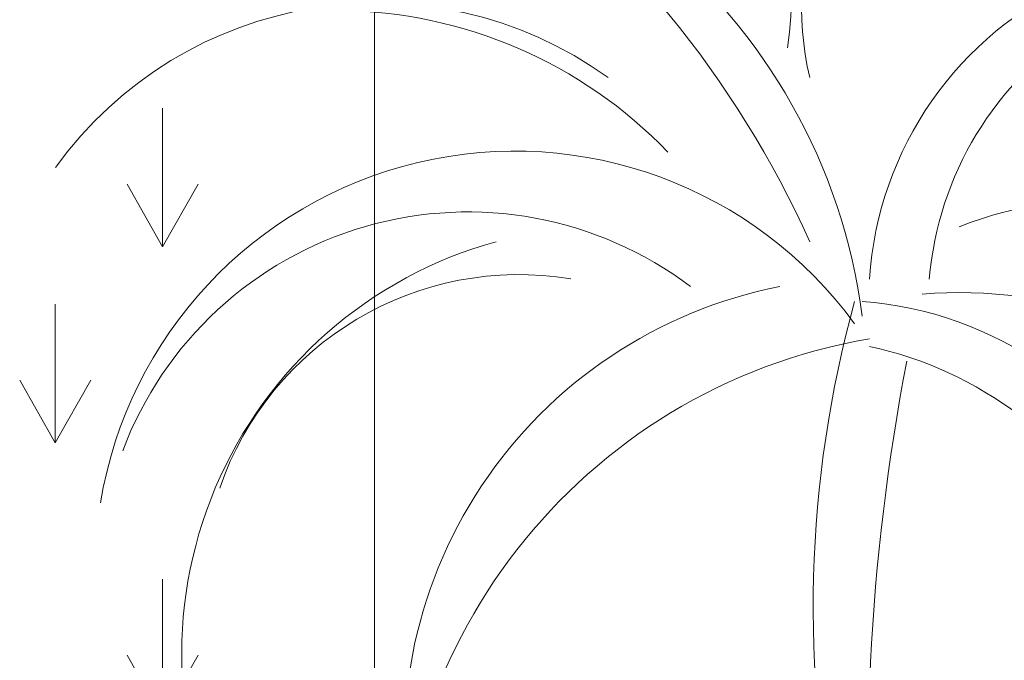
# Model space of a CAD drawing. Units: millimetres. Extents: x 595116 to 630915, y 909473 to 920225.
# Tile 108 of 134: x 629792 to 629817, y 919201 to 919217. Entities that reach past the tile are written whole.
import ezdxf

# ---------------------------------------------------------------- set-up
doc = ezdxf.new("R2010")
doc.units = ezdxf.units.MM
doc.layers.add('L-PLNT', color=85, linetype='Continuous', lineweight=13)

# ---------------------------------------------------------------- blocks, each defined once
blk = doc.blocks.new('tree')
for centre, radius, start, end in [((629595.141, 919296.95), 5.184, 352.032, 57.0714), ((629604.232, 919296.737), 3.791, 61.1347, 193.108), ((629594.259, 919292.132), 6.965, 7.4001, 94.0059), ((629589.446, 919288.922), 12.167, 24.2477, 54.3726), ((629605.429, 919293.205), 4.185, 348.9977, 176.315), ((629605.915, 919293.144), 3.963, 69.3845, 175.231), ((629595.377, 919292.044), 4.722, 54.2484, 144.2167), ((629594.88, 919291.171), 5.506, 43.8672, 89.4805), ((629597.025, 919289.989), 5.01, 36.0581, 170.6542), ((629596.464, 919289.874), 4.4, 52.9074, 159.3471), ((629603.809, 919290.469), 3.92, 343.886, 112.2662), ((629598.153, 919288.998), 5.103, 105.3576, 208.8973), ((629597.068, 919289.758), 3.768, 80.4816, 161.0664), ((629601.247, 919287.941), 5.545, 101.0419, 191.8692), ((629602.329, 919287.957), 5.355, 355.2141, 94.8217), ((629614.329, 919289.554), 13.748, 164.5925, 192.323), ((629600.849, 919288.894), 4.324, 322.5461, 85.805), ((629602.391, 919286.088), 6.769, 99.681, 184.5451), ((629600.275, 919288.191), 4.585, 338.7925, 77.6921), ((629626.813, 919287.645), 25.579, 169.0753, 185.2889)]:
    blk.add_arc(centre, radius, start, end)
blk = doc.blocks.new('LAWN-GRASS-TUFT')
blk.add_line((0.892, 3.485), (0.892, 0))
blk.add_lwpolyline([(0, 1.577), (0.892, 0), (1.785, 1.577)])

msp = doc.modelspace()

# ---------------------------------------------------------------- linework, layer by layer
at = {"layer": 'L-PLNT'}
msp.add_line((629800.951, 919184.917), (629800.951, 919266.009), dxfattribs=at)

# ---------------------------------------------------------------- block references
at = {"layer": 'L-PLNT', "xscale": 2.107689410566463, "yscale": 2.107689410566463, "zscale": 2.107689410566463}
msp.add_blockref('tree', (-697190.499, -1018374.553), dxfattribs=at)
at = {"layer": 'L-PLNT'}
for p in [(629794.733, 919211.374), (629792.034, 919206.447), (629794.733, 919199.536)]:
    msp.add_blockref('LAWN-GRASS-TUFT', p, dxfattribs=at)

doc.saveas('drawing.dxf')
